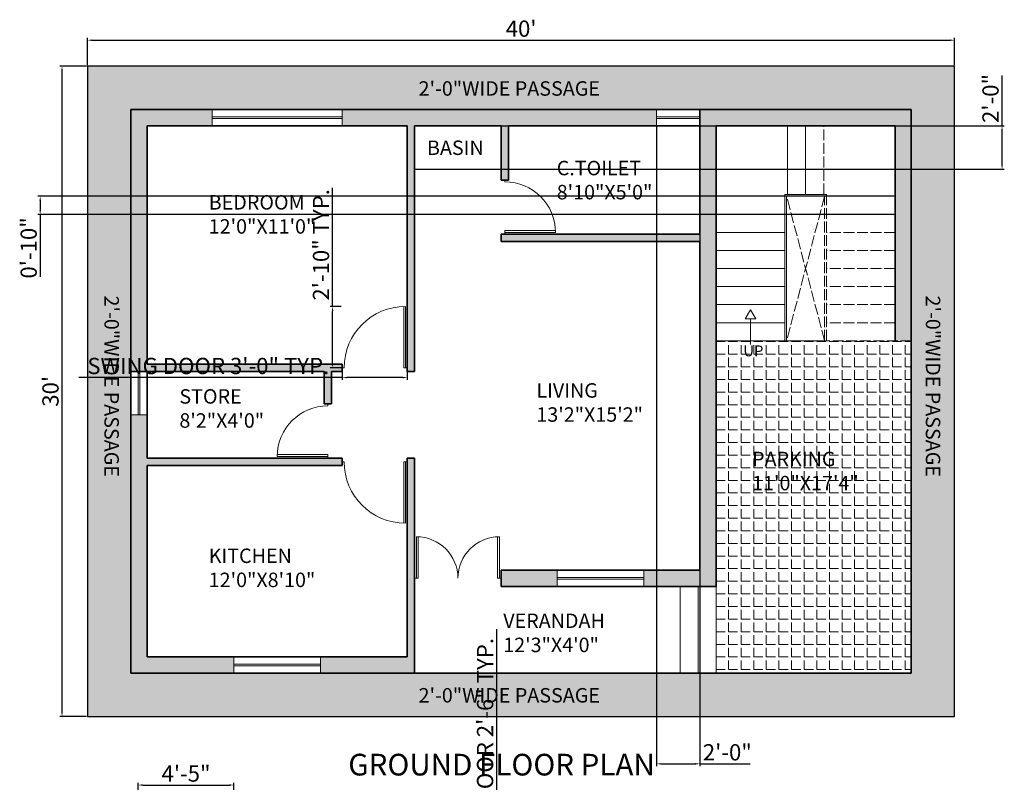
# Model space of a CAD drawing. Units: inches. Extents: x 1947 to 4744, y 610 to 1869.
# Tile 7 of 8: x 3652 to 4197, y 1446 to 1869. Entities that reach past the tile are written whole.
import ezdxf

# ---------------------------------------------------------------- set-up
doc = ezdxf.new("R2010")
doc.units = ezdxf.units.IN
doc.linetypes.add('ACAD_ISO02W100', pattern=[15, 12, -3])
for name, color, linetype, lineweight in [('A-ANNO-DIMS', 2, 'Continuous', 18), ('A-ANNO-SYMB', 2, 'Continuous', 18), ('A-ANNO-TEXT', 7, 'Continuous', 18), ('A-ANNO-TITL', 7, 'Continuous', 35), ('A-AREA-IDEN', 7, 'Continuous', 18), ('A-DOOR', 3, 'Continuous', 18), ('A-FLOR-FIXT', 9, 'Continuous', 18), ('A-FLOR-STRS', 7, 'Continuous', 18), ('A-FLOR-STRS-OVHD', 7, 'ACAD_ISO02W100', 13), ('A-GLAZ', 4, 'Continuous', 18), ('A-WALL', 7, 'Continuous', 35), ('C-PROP', 8, 'Continuous', 25)]:
    doc.layers.add(name, color=color, linetype=linetype, lineweight=lineweight)
doc.layers.add('A-FLOR-PATT', color=251, linetype='Continuous', lineweight=13, true_color=0x636466)
doc.layers.add('A-WALL-PATT', color=18, linetype='Continuous', lineweight=13, true_color=0x000000)
doc.styles.get("Standard").update_dxf_attribs({"font": 'arial.ttf'})
doc.dimstyles.new('ISO-25', dxfattribs={"dimtxt": 9, "dimasz": 2.5, "dimexe": 1.25, "dimexo": 0.625, "dimtad": 1, "dimdec": 1, "dimlunit": 3, "dimtxsty": 'Standard', "dimcen": 2.5, "dimadec": 0, "dimazin": 0, "dimtfac": 1, "dimtdec": 1, "dimtmove": 0, "dimatfit": 3, "dimfxl": 1, "dimarcsym": 0})
pattern_1 = [(0, (0, 0), (0, 6.985), [5.08, -1.905]), (90, (0, 0), (-6.985, 4e-16), [5.08, -1.905])]

# ---------------------------------------------------------------- blocks, each defined once
blk = doc.blocks.new('1')
for p, q in [((4267.36, 1627.82), (4267.36, 1650.82)), ((4268.36, 1627.82), (4268.36, 1650.82)), ((4312.36, 1627.82), (4312.36, 1650.82)), ((4313.36, 1627.82), (4313.36, 1650.82)), ((4266.36, 1627.82), (4268.36, 1627.82)), ((4314.36, 1627.82), (4312.36, 1627.82))]:
    blk.add_line(p, q)
at = {"ltscale": 0.5}
for centre, start, end in [((4267.36, 1627.82), 0, 90), ((4313.36, 1627.82), 90, 180)]:
    blk.add_arc(centre, 23, start, end, dxfattribs=at)
blk = doc.blocks.new('2')
for p, q in [((4319.45, 1679.18), (4319.45, 1713.18)), ((4320.45, 1679.18), (4320.45, 1713.18)), ((4318.45, 1679.18), (4320.45, 1679.18)), ((4353.45, 1679.18), (4354.45, 1679.18))]:
    blk.add_line(p, q)
at = {"ltscale": 0.5}
blk.add_arc((4319.45, 1679.18), 34, 0, 90, dxfattribs=at)
blk = doc.blocks.new('4')
for p, q in [((3808.6, 1693.11), (3808.6, 1721.11)), ((3809.6, 1693.11), (3809.6, 1721.11)), ((3807.6, 1693.11), (3809.6, 1693.11)), ((3836.6, 1693.11), (3837.6, 1693.11))]:
    blk.add_line(p, q)
at = {"ltscale": 0.5}
blk.add_arc((3808.6, 1693.11), 28, 0, 90, dxfattribs=at)
blk = doc.blocks.new('*D5')
at = {"layer": 'A-ANNO-DIMS', "color": 0, "lineweight": -2, "transparency": 16777216}
for p, q in [((3688.91, 1842.83), (3674.11, 1842.83)), ((3675.36, 1485.33), (3675.36, 1840.33)), ((3688.91, 1482.83), (3674.11, 1482.83))]:
    blk.add_line(p, q, dxfattribs=at)
at = {"layer": 'A-ANNO-DIMS', "color": 0, "transparency": 16777216}
for points in [[(3674.94, 1840.33), (3675.78, 1840.33), (3675.36, 1842.83)], [(3674.94, 1485.33), (3675.78, 1485.33), (3675.36, 1482.83)]]:
    blk.add_solid(points, dxfattribs=at)
at = {"layer": 'Defpoints', "color": 0, "transparency": 16777216}
for p in [(3675.36, 1842.83), (3689.53, 1842.83), (3689.53, 1482.83)]:
    blk.add_point(p, dxfattribs=at)
at = {"layer": 'A-ANNO-DIMS', "color": 0, "transparency": 16777216, "insert": (3670.14, 1662.83), "char_height": 9, "attachment_point": 5, "rotation": 90}
blk.add_mtext("30'", dxfattribs=at)
blk = doc.blocks.new('*D6')
at = {"layer": 'A-ANNO-DIMS', "color": 0, "lineweight": -2, "transparency": 16777216}
for p, q in [((3689.53, 1843.45), (3689.53, 1858.52)), ((3692.03, 1857.27), (4167.03, 1857.27)), ((4169.53, 1843.45), (4169.53, 1858.52))]:
    blk.add_line(p, q, dxfattribs=at)
at = {"layer": 'A-ANNO-DIMS', "color": 0, "transparency": 16777216}
for points in [[(3692.03, 1857.68), (3692.03, 1856.85), (3689.53, 1857.27)], [(4167.03, 1857.68), (4167.03, 1856.85), (4169.53, 1857.27)]]:
    blk.add_solid(points, dxfattribs=at)
at = {"layer": 'Defpoints', "color": 0, "transparency": 16777216}
for p in [(4169.53, 1857.27), (3689.53, 1842.83), (4169.53, 1842.83)]:
    blk.add_point(p, dxfattribs=at)
at = {"layer": 'A-ANNO-DIMS', "color": 0, "transparency": 16777216, "insert": (3929.53, 1862.49), "char_height": 9, "attachment_point": 5}
blk.add_mtext("40'", dxfattribs=at)
blk = doc.blocks.new('STAIR-DIRECTION')
blk.add_line((2.91, 14.18), (2.91, 0))
blk.add_lwpolyline([(2.91, 19.23), (0, 14.18), (5.83, 14.18)], close=True)
blk = doc.blocks.new('*D80')
at = {"layer": 'A-ANNO-DIMS', "color": 0, "lineweight": -2, "transparency": 16777216}
for p, q in [((3830.53, 1675.2), (3830.53, 1669.18)), ((3866.53, 1675.2), (3866.53, 1669.18)), ((3830.53, 1670.43), (3684.65, 1670.43)), ((3864.03, 1670.43), (3833.03, 1670.43))]:
    blk.add_line(p, q, dxfattribs=at)
at = {"layer": 'A-ANNO-DIMS', "color": 0, "transparency": 16777216}
for points in [[(3833.03, 1670.84), (3833.03, 1670.01), (3830.53, 1670.43)], [(3864.03, 1670.84), (3864.03, 1670.01), (3866.53, 1670.43)]]:
    blk.add_solid(points, dxfattribs=at)
at = {"layer": 'Defpoints', "color": 0, "transparency": 16777216}
for p in [(3830.53, 1675.83), (3866.53, 1675.83), (3830.53, 1670.43)]:
    blk.add_point(p, dxfattribs=at)
at = {"layer": 'A-ANNO-DIMS', "color": 0, "transparency": 16777216, "insert": (3756.34, 1675.71), "char_height": 9, "attachment_point": 5}
blk.add_mtext('SWING DOOR 3\'-0" TYP.', dxfattribs=at)
blk = doc.blocks.new('*D81')
at = {"layer": 'A-ANNO-DIMS', "color": 0, "lineweight": -2, "transparency": 16777216}
for p, q in [((3825.13, 1709.83), (3825.13, 1775.58)), ((3829.91, 1709.83), (3823.88, 1709.83)), ((3825.13, 1678.33), (3825.13, 1707.33)), ((3829.91, 1675.83), (3823.88, 1675.83))]:
    blk.add_line(p, q, dxfattribs=at)
at = {"layer": 'A-ANNO-DIMS', "color": 0, "transparency": 16777216}
for points in [[(3824.71, 1707.33), (3825.55, 1707.33), (3825.13, 1709.83)], [(3824.71, 1678.33), (3825.55, 1678.33), (3825.13, 1675.83)]]:
    blk.add_solid(points, dxfattribs=at)
at = {"layer": 'Defpoints', "color": 0, "transparency": 16777216}
for p in [(3825.13, 1709.83), (3830.53, 1709.83), (3830.53, 1675.83)]:
    blk.add_point(p, dxfattribs=at)
at = {"layer": 'A-ANNO-DIMS', "color": 0, "transparency": 16777216, "insert": (3819.91, 1743.96), "char_height": 9, "attachment_point": 5, "rotation": 90}
blk.add_mtext('2\'-10" TYP.', dxfattribs=at)
blk = doc.blocks.new('*D82')
at = {"layer": 'A-ANNO-DIMS', "color": 0, "lineweight": -2, "transparency": 16777216}
for p, q in [((3916.03, 1381.79), (3916.03, 1531.18)), ((3919.91, 1381.79), (3914.78, 1381.79)), ((3916.03, 1354.29), (3916.03, 1379.29)), ((3919.91, 1351.79), (3914.78, 1351.79))]:
    blk.add_line(p, q, dxfattribs=at)
at = {"layer": 'A-ANNO-DIMS', "color": 0, "transparency": 16777216}
for points in [[(3915.61, 1379.29), (3916.45, 1379.29), (3916.03, 1381.79)], [(3915.61, 1354.29), (3916.45, 1354.29), (3916.03, 1351.79)]]:
    blk.add_solid(points, dxfattribs=at)
at = {"layer": 'Defpoints', "color": 0, "transparency": 16777216}
for p in [(3916.03, 1381.79), (3920.53, 1381.79), (3920.53, 1351.79)]:
    blk.add_point(p, dxfattribs=at)
at = {"layer": 'A-ANNO-DIMS', "color": 0, "transparency": 16777216, "insert": (3910.75, 1457.73), "char_height": 9, "attachment_point": 5, "rotation": 90}
blk.add_mtext('SINGLE DOOR 2\'-6" TYP.', dxfattribs=at)
blk = doc.blocks.new('*D98')
at = {"layer": 'A-ANNO-DIMS', "color": 0, "lineweight": -2, "transparency": 16777216}
for p, q in [((4135.91, 1770.83), (3662.03, 1770.83)), ((3663.28, 1768.33), (3663.28, 1763.33)), ((4135.91, 1760.83), (3662.03, 1760.83)), ((3663.28, 1760.83), (3663.28, 1726.16))]:
    blk.add_line(p, q, dxfattribs=at)
at = {"layer": 'A-ANNO-DIMS', "color": 0, "transparency": 16777216}
for points in [[(3662.86, 1768.33), (3663.7, 1768.33), (3663.28, 1770.83)], [(3662.86, 1763.33), (3663.7, 1763.33), (3663.28, 1760.83)]]:
    blk.add_solid(points, dxfattribs=at)
at = {"layer": 'Defpoints', "color": 0, "transparency": 16777216}
for p in [(4136.53, 1770.83), (3663.28, 1760.83), (4136.53, 1760.83)]:
    blk.add_point(p, dxfattribs=at)
at = {"layer": 'A-ANNO-DIMS', "color": 0, "transparency": 16777216, "insert": (3658.06, 1742.24), "char_height": 9, "attachment_point": 5, "rotation": 90}
blk.add_mtext('0\'-10"', dxfattribs=at)
blk = doc.blocks.new('*D100')
at = {"layer": 'A-ANNO-DIMS', "color": 0, "lineweight": -2, "transparency": 16777216}
for p, q in [((4195.78, 1809.83), (4195.78, 1837.66)), ((3871.16, 1809.83), (4197.03, 1809.83)), ((4195.78, 1788.33), (4195.78, 1807.33)), ((3871.16, 1785.83), (4197.03, 1785.83))]:
    blk.add_line(p, q, dxfattribs=at)
at = {"layer": 'A-ANNO-DIMS', "color": 0, "transparency": 16777216}
for points in [[(4195.36, 1807.33), (4196.2, 1807.33), (4195.78, 1809.83)], [(4195.36, 1788.33), (4196.2, 1788.33), (4195.78, 1785.83)]]:
    blk.add_solid(points, dxfattribs=at)
at = {"layer": 'Defpoints', "color": 0, "transparency": 16777216}
for p in [(3870.53, 1809.83), (4195.78, 1809.83), (3870.53, 1785.83)]:
    blk.add_point(p, dxfattribs=at)
at = {"layer": 'A-ANNO-DIMS', "color": 0, "transparency": 16777216, "insert": (4190.56, 1824.99), "char_height": 9, "attachment_point": 5, "rotation": 90}
blk.add_mtext('2\'-0"', dxfattribs=at)
blk = doc.blocks.new('*D108')
at = {"layer": 'A-ANNO-DIMS', "color": 0, "lineweight": -2, "transparency": 16777216}
for p, q in [((3717.53, 1113.41), (3717.53, 1446.09)), ((3720.03, 1444.84), (3768.03, 1444.84)), ((3770.53, 1113.41), (3770.53, 1446.09))]:
    blk.add_line(p, q, dxfattribs=at)
at = {"layer": 'A-ANNO-DIMS', "color": 0, "transparency": 16777216}
for points in [[(3720.03, 1445.26), (3720.03, 1444.42), (3717.53, 1444.84)], [(3768.03, 1445.26), (3768.03, 1444.42), (3770.53, 1444.84)]]:
    blk.add_solid(points, dxfattribs=at)
at = {"layer": 'Defpoints', "color": 0, "transparency": 16777216}
for p in [(3770.53, 1444.84), (3717.53, 1112.79), (3770.53, 1112.79)]:
    blk.add_point(p, dxfattribs=at)
at = {"layer": 'A-ANNO-DIMS', "color": 0, "transparency": 16777216, "insert": (3744.03, 1450.04), "char_height": 9, "attachment_point": 5}
blk.add_mtext('4\'-5"', dxfattribs=at)
blk = doc.blocks.new('*D112')
at = {"layer": 'A-ANNO-DIMS', "color": 0, "lineweight": -2, "transparency": 16777216}
for p, q in [((4004.53, 1809.2), (4004.53, 1455.33)), ((4028.53, 1809.2), (4028.53, 1455.33)), ((4007.03, 1456.58), (4026.03, 1456.58)), ((4028.53, 1456.58), (4056.36, 1456.58))]:
    blk.add_line(p, q, dxfattribs=at)
at = {"layer": 'A-ANNO-DIMS', "color": 0, "transparency": 16777216}
for points in [[(4007.03, 1456.99), (4007.03, 1456.16), (4004.53, 1456.58)], [(4026.03, 1456.99), (4026.03, 1456.16), (4028.53, 1456.58)]]:
    blk.add_solid(points, dxfattribs=at)
at = {"layer": 'Defpoints', "color": 0, "transparency": 16777216}
for p in [(4004.53, 1809.83), (4028.53, 1809.83), (4028.53, 1456.58)]:
    blk.add_point(p, dxfattribs=at)
at = {"layer": 'A-ANNO-DIMS', "color": 0, "transparency": 16777216, "insert": (4043.69, 1461.8), "char_height": 9, "attachment_point": 5}
blk.add_mtext('2\'-0"', dxfattribs=at)

msp = doc.modelspace()

# ---------------------------------------------------------------- hatches: boundary and pattern name
at = {"layer": 'A-FLOR-PATT'}
h = msp.add_hatch(dxfattribs=at)
h.set_pattern_fill('ANGLE', color=256)
h.set_pattern_definition(pattern_1)
h.paths.add_polyline_path([(3689.53, 1842.83), (3689.53, 1482.83), (4169.53, 1482.83), (4169.53, 1842.83)])
h.paths.add_polyline_path([(4145.53, 1818.83), (4145.53, 1506.83), (3713.53, 1506.83), (3713.53, 1818.83)], flags=16)
h.paths.add_polyline_path([(4136.53, 1809.83), (4136.53, 1690.83), (4097.53, 1690.83), (4037.53, 1690.83), (4037.53, 1554.83), (3918.53, 1554.83), (3918.53, 1563.83), (4028.53, 1563.83), (4028.53, 1745.83), (3918.53, 1745.83), (3918.53, 1749.83), (4028.53, 1749.83), (4028.53, 1809.83), (3922.53, 1809.83), (3922.53, 1779.83), (3918.53, 1779.83), (3918.53, 1785.83), (3870.53, 1785.83), (3870.53, 1673.83), (3866.53, 1673.83), (3866.53, 1809.83), (3722.53, 1809.83), (3722.53, 1677.83), (3830.53, 1677.83), (3830.53, 1673.83), (3824.53, 1673.83), (3824.53, 1655.83), (3820.53, 1655.83), (3820.53, 1673.83), (3722.53, 1673.83), (3722.53, 1625.83), (3830.53, 1625.83), (3830.53, 1621.83), (3722.53, 1621.83), (3722.53, 1515.83), (3818.53, 1515.83), (3818.53, 1510.83), (3770.53, 1510.83), (3770.53, 1515.83), (3722.53, 1515.83), (3722.53, 1621.83), (3830.53, 1621.83), (3830.53, 1625.83), (3722.53, 1625.83), (3722.53, 1649.83), (3717.53, 1649.83), (3717.53, 1673.83), (3820.53, 1673.83), (3820.53, 1655.83), (3824.53, 1655.83), (3824.53, 1673.83), (3830.53, 1673.83), (3830.53, 1677.83), (3722.53, 1677.83), (3722.53, 1809.83), (3758.53, 1809.83), (3758.53, 1814.83), (3830.53, 1814.83), (3830.53, 1809.83), (3866.53, 1809.83), (3866.53, 1673.83), (3870.53, 1673.83), (3870.53, 1809.83), (3918.53, 1809.83), (3918.53, 1779.83), (3922.53, 1779.83), (3922.53, 1809.83), (4004.53, 1809.83), (4004.53, 1814.83), (4028.53, 1814.83), (4028.53, 1749.83), (3918.53, 1749.83), (3918.53, 1745.83), (4028.53, 1745.83), (4028.53, 1563.83), (3997.53, 1563.83), (3997.53, 1554.83), (4037.53, 1554.83), (4037.53, 1809.83)], flags=0)
h.paths.add_polyline_path([(4076.53, 1770.83), (4097.53, 1770.83), (4097.53, 1690.83), (4087.03, 1730.83), (4076.53, 1690.83)], flags=0)
h.paths.add_polyline_path([(3875.22, 1789.16), (3914.67, 1789.16), (3914.67, 1806.24), (3875.22, 1806.24)], flags=8)
h.paths.add_polyline_path([(3870.52, 1485.98), (3983.52, 1485.98), (3983.52, 1503.06), (3870.52, 1503.06)], flags=24)
h.paths.add_polyline_path([(3694.29, 1718.11), (3694.29, 1605.12), (3711.37, 1605.12), (3711.37, 1718.11)], flags=24)
h.paths.add_polyline_path([(4149.02, 1718.11), (4149.02, 1605.12), (4166.11, 1605.12), (4166.11, 1718.11)], flags=24)
h.paths.add_polyline_path([(3870.52, 1821.98), (3983.52, 1821.98), (3983.52, 1839.06), (3870.52, 1839.06)], flags=24)
h.paths.add_polyline_path([(3916.25, 1513.88), (3987.81, 1513.88), (3987.81, 1544.29), (3916.25, 1544.29)], flags=8)
h.paths.add_polyline_path([(4054.04, 1603.48), (4115.91, 1603.48), (4115.91, 1633.9), (4054.04, 1633.9)], flags=8)
h.paths.add_polyline_path([(3737.61, 1638.13), (3787.69, 1638.13), (3787.69, 1668.55), (3737.61, 1668.55)], flags=8)
h.paths.add_polyline_path([(3946.51, 1764.58), (4002.96, 1764.58), (4002.96, 1795), (3946.51, 1795)], flags=8)
h.paths.add_polyline_path([(3934.6, 1641.45), (3996.46, 1641.45), (3996.46, 1671.86), (3934.6, 1671.86)], flags=8)
h.paths.add_polyline_path([(3753.2, 1549.89), (3815.06, 1549.89), (3815.06, 1580.3), (3753.2, 1580.3)], flags=8)
h.paths.add_polyline_path([(3753.2, 1745.59), (3817.45, 1745.59), (3817.45, 1776), (3753.2, 1776)], flags=8)
h = msp.add_hatch(dxfattribs=at)
h.set_pattern_fill('ANGLE', color=256)
h.set_pattern_definition(pattern_1)
h.paths.add_polyline_path([(4145.53, 1690.83), (4097.53, 1690.83), (4037.53, 1690.83), (4037.53, 1554.83), (4037.53, 1506.83), (4145.53, 1506.83)])
h.paths.add_polyline_path([(4051, 1678.84), (4065.33, 1678.84), (4065.33, 1691.65), (4051, 1691.65)], flags=9)
h.paths.add_polyline_path([(4054.04, 1603.48), (4115.91, 1603.48), (4115.91, 1633.9), (4054.04, 1633.9)], flags=24)
at = {"layer": 'A-WALL-PATT'}
h = msp.add_hatch(color=256, dxfattribs=at)
h.dxf.hatch_style = 1
h.paths.add_polyline_path([(3758.53, 1818.83), (3713.53, 1818.83), (3713.53, 1673.83), (3820.53, 1673.83), (3820.53, 1655.83), (3824.53, 1655.83), (3824.53, 1673.83), (3830.53, 1673.83), (3830.53, 1677.83), (3722.53, 1677.83), (3722.53, 1809.83), (3758.53, 1809.83)])
h.paths.add_polyline_path([(4004.53, 1818.83), (3830.53, 1818.83), (3830.53, 1809.83), (3866.53, 1809.83), (3866.53, 1673.83), (3870.53, 1673.83), (3870.53, 1809.83), (3918.53, 1809.83), (3918.53, 1779.83), (3922.53, 1779.83), (3922.53, 1809.83), (4004.53, 1809.83)])
h.paths.add_polyline_path([(4037.53, 1809.83), (4136.53, 1809.83), (4136.53, 1690.83), (4145.53, 1690.83), (4145.53, 1818.83), (4028.53, 1818.83), (4028.53, 1749.83), (3918.53, 1749.83), (3918.53, 1745.83), (4028.53, 1745.83), (4028.53, 1563.83), (3997.53, 1563.83), (3997.53, 1554.83), (4037.53, 1554.83)])
h.paths.add_polyline_path([(3870.53, 1625.83), (3866.53, 1625.83), (3866.53, 1515.83), (3818.53, 1515.83), (3818.53, 1506.83), (3870.53, 1506.83)])
h.paths.add_polyline_path([(3770.53, 1515.83), (3722.53, 1515.83), (3722.53, 1621.83), (3830.53, 1621.83), (3830.53, 1625.83), (3722.53, 1625.83), (3722.53, 1649.83), (3713.53, 1649.83), (3713.53, 1506.83), (3770.53, 1506.83)])
h.paths.add_polyline_path([(3949.53, 1563.83), (3918.53, 1563.83), (3918.53, 1554.83), (3949.53, 1554.83)])

# ---------------------------------------------------------------- linework, layer by layer
at = {"layer": 'A-FLOR-FIXT'}
msp.add_line((3918.53, 1785.83), (3870.53, 1785.83), dxfattribs=at)
at = {"layer": 'A-FLOR-STRS'}
for p, q in [((4077.03, 1771.83), (4077.03, 1809.83)), ((4087.03, 1771.83), (4087.03, 1809.83)), ((4098.53, 1771.83), (4075.53, 1771.83)), ((4075.53, 1690.83), (4075.53, 1771.83)), ((4075.53, 1770.83), (4037.53, 1770.83)), ((4097.53, 1770.83), (4076.53, 1770.83)), ((4076.53, 1690.83), (4076.53, 1770.83)), ((4075.53, 1760.83), (4037.53, 1760.83)), ((4075.53, 1750.83), (4037.53, 1750.83)), ((4075.53, 1740.83), (4037.53, 1740.83)), ((4075.53, 1730.83), (4037.53, 1730.83)), ((4075.53, 1720.83), (4037.53, 1720.83)), ((4075.53, 1710.83), (4037.53, 1710.83)), ((4075.53, 1700.83), (4037.53, 1700.83)), ((4097.53, 1690.83), (4037.53, 1690.83)), ((4017.53, 1554.83), (4017.53, 1506.83)), ((4027.53, 1554.83), (4027.53, 1506.83)), ((4037.53, 1554.83), (4037.53, 1506.83))]:
    msp.add_line(p, q, dxfattribs=at)
at = {"layer": 'A-FLOR-STRS-OVHD', "ltscale": 0.5}
for p, q in [((4097.03, 1771.83), (4097.03, 1809.83)), ((4098.53, 1690.83), (4098.53, 1771.83)), ((4097.53, 1770.83), (4076.53, 1690.83)), ((4097.53, 1690.83), (4076.53, 1770.83)), ((4097.53, 1690.83), (4097.53, 1770.83)), ((4136.53, 1770.83), (4098.53, 1770.83)), ((4136.53, 1760.83), (4098.53, 1760.83)), ((4136.53, 1750.83), (4098.53, 1750.83)), ((4136.53, 1740.83), (4098.53, 1740.83)), ((4136.53, 1730.83), (4098.53, 1730.83)), ((4136.53, 1720.83), (4098.53, 1720.83)), ((4136.53, 1710.83), (4098.53, 1710.83)), ((4136.53, 1700.83), (4098.53, 1700.83)), ((4145.53, 1690.83), (4097.53, 1690.83))]:
    msp.add_line(p, q, dxfattribs=at)
at = {"layer": 'A-GLAZ'}
for p, q in [((3758.53, 1809.83), (3758.53, 1818.83)), ((3830.53, 1809.83), (3830.53, 1818.83)), ((4004.53, 1809.83), (4004.53, 1818.83)), ((3830.53, 1814.83), (3758.53, 1814.83)), ((3830.53, 1813.83), (3758.53, 1813.83)), ((4028.53, 1814.83), (4004.53, 1814.83)), ((4028.53, 1813.83), (4004.53, 1813.83)), ((3717.53, 1673.83), (3717.53, 1649.83)), ((3718.53, 1673.83), (3718.53, 1649.83)), ((3722.53, 1649.83), (3713.53, 1649.83)), ((3949.53, 1554.83), (3949.53, 1563.83)), ((3997.53, 1559.83), (3949.53, 1559.83)), ((3997.53, 1554.83), (3997.53, 1563.83)), ((3997.53, 1558.83), (3949.53, 1558.83)), ((3770.53, 1506.83), (3770.53, 1515.83)), ((3818.53, 1506.83), (3818.53, 1515.83)), ((3818.53, 1511.83), (3770.53, 1511.83)), ((3818.53, 1510.83), (3770.53, 1510.83))]:
    msp.add_line(p, q, dxfattribs=at)
at = {"layer": 'A-WALL'}
for p, q in [((4145.53, 1818.83), (3713.53, 1818.83)), ((3713.53, 1818.83), (3713.53, 1506.83)), ((4028.53, 1749.83), (4028.53, 1818.83)), ((4145.53, 1506.83), (4145.53, 1818.83)), ((3722.53, 1809.83), (3722.53, 1677.83)), ((3866.53, 1809.83), (3722.53, 1809.83)), ((3866.53, 1809.83), (3866.53, 1673.83)), ((3870.53, 1809.83), (3870.53, 1673.83)), ((3918.53, 1809.83), (3870.53, 1809.83)), ((3918.53, 1779.83), (3918.53, 1809.83)), ((3922.53, 1779.83), (3922.53, 1809.83)), ((4028.53, 1809.83), (3922.53, 1809.83)), ((4136.53, 1809.83), (4037.53, 1809.83)), ((4037.53, 1554.83), (4037.53, 1809.83)), ((4136.53, 1690.83), (4136.53, 1809.83)), ((3922.53, 1779.83), (3918.53, 1779.83)), ((4028.53, 1749.83), (3918.53, 1749.83)), ((3918.53, 1745.83), (3918.53, 1749.83)), ((3918.53, 1745.83), (4028.53, 1745.83)), ((4028.53, 1563.83), (4028.53, 1745.83)), ((3820.53, 1673.83), (3713.53, 1673.83)), ((3830.53, 1677.83), (3722.53, 1677.83)), ((3722.53, 1673.83), (3722.53, 1625.83)), ((3820.53, 1673.83), (3820.53, 1655.83)), ((3824.53, 1673.83), (3824.53, 1655.83)), ((3830.53, 1673.83), (3824.53, 1673.83)), ((3830.53, 1677.83), (3830.53, 1673.83)), ((3870.53, 1673.83), (3866.53, 1673.83)), ((3824.53, 1655.83), (3820.53, 1655.83)), ((3830.53, 1625.83), (3722.53, 1625.83)), ((3830.53, 1625.83), (3830.53, 1621.83)), ((3870.53, 1625.83), (3866.53, 1625.83)), ((3866.53, 1625.83), (3866.53, 1515.83)), ((3870.53, 1625.83), (3870.53, 1506.83)), ((3830.53, 1621.83), (3722.53, 1621.83)), ((3722.53, 1621.83), (3722.53, 1515.83)), ((3918.53, 1563.83), (4028.53, 1563.83)), ((3918.53, 1563.83), (3918.53, 1554.83)), ((3918.53, 1554.83), (4037.53, 1554.83)), ((3722.53, 1515.83), (3866.53, 1515.83)), ((3713.53, 1506.83), (4145.53, 1506.83))]:
    msp.add_line(p, q, dxfattribs=at)
at = {"layer": 'C-PROP'}
msp.add_lwpolyline([(3689.53, 1482.83), (4169.53, 1482.83), (4169.53, 1842.83), (3689.53, 1842.83)], close=True, dxfattribs=at)

# ---------------------------------------------------------------- block references
at = {"layer": 'A-ANNO-SYMB'}
msp.add_blockref('STAIR-DIRECTION', (4053.62, 1688.75), dxfattribs=at)
at = {"layer": 'A-DOOR', "xscale": -1, "rotation": 270}
msp.add_blockref('4', (2227.42, -2057.77), dxfattribs=at)
at = {"layer": 'A-DOOR', "xscale": -1}
msp.add_blockref('2', (8184.98, -3.36), dxfattribs=at)
at = {"layer": 'A-DOOR'}
for name, p, rotation in [('4', (5515.64, -2181.77), 90), ('2', (8184.98, 3303.01), 180)]:
    msp.add_blockref(name, p, dxfattribs=dict(at, rotation=rotation))
msp.add_blockref('1', (-395.83, -68.5), dxfattribs=at)

# ---------------------------------------------------------------- texts
at = {"layer": 'A-ANNO-TEXT', "attachment_point": 1}
for s, insert, char_height in [('{\\fTimes New Roman|b0|i0|c0|p18;BASIN}', (3877.42, 1801.71), 8), ('{\\fTimes New Roman|b0|i0|c0|p18;UP}', (4052.55, 1688.25), 6)]:
    msp.add_mtext_dynamic_manual_height_columns(s, width=158.3328, gutter_width=12.5, heights=[0], dxfattribs=dict(at, insert=insert, char_height=char_height))
at = {"layer": 'A-ANNO-TITL', "insert": (3833.83, 1462.13), "char_height": 12, "attachment_point": 1}
msp.add_mtext_dynamic_manual_height_columns('{\\fTimes New Roman|b0|i0|c0|p18;GROUND FLOOR PLAN}', width=253.4596, gutter_width=12.5, heights=[0], dxfattribs=at)
at = {"layer": 'A-AREA-IDEN', "char_height": 8, "attachment_point": 1}
for s, width, heights, insert in [('{\\fTimes New Roman|b0|i0|c0|p18;2\'-0"WIDE PASSAGE}', 158.3328, [0], (3872.77, 1834.53)), ('{\\fTimes New Roman|b0|i0|c0|p18;C.TOILET\\P8\'10"X5\'0"}', 64.3566, [21.47], (3949.23, 1790.47)), ('{\\fTimes New Roman|b0|i0|c0|p18;BEDROOM\\P12\'0"X11\'0"}', 64.3566, [0], (3756.58, 1771.48)), ('{\\fTimes New Roman|b0|i0|c0|p18;STORE\\P8\'2"X4\'0"}', 64.3566, [21.47], (3740.35, 1664.02)), ('{\\fTimes New Roman|b0|i0|c0|p18;LIVING\\P13\'2"X15\'2"}', 64.3566, [21.47], (3937.98, 1667.33)), ('{\\fTimes New Roman|b0|i0|c0|p18;PARKING\\P11\'0"X17\'4"}', 64.3566, [0], (4057.42, 1629.37)), ('{\\fTimes New Roman|b0|i0|c0|p18;KITCHEN\\P12\'0"X8\'10"}', 64.3566, [0], (3756.58, 1575.78)), ('{\\fTimes New Roman|b0|i0|c0|p18;VERANDAH\\P12\'3"X4\'0"}', 64.3566, [0], (3919.64, 1539.77)), ('{\\fTimes New Roman|b0|i0|c0|p18;2\'-0"WIDE PASSAGE}', 158.3328, [0], (3872.77, 1498.53))]:
    msp.add_mtext_dynamic_manual_height_columns(s, width=width, gutter_width=12.5, heights=heights, dxfattribs=dict(at, insert=insert))
at = {"layer": 'A-AREA-IDEN', "char_height": 8, "attachment_point": 1, "rotation": 270}
for insert in [(3706.84, 1715.86), (4161.58, 1715.86)]:
    msp.add_mtext_dynamic_manual_height_columns('{\\fTimes New Roman|b0|i0|c0|p18;2\'-0"WIDE PASSAGE}', width=158.3328, gutter_width=12.5, heights=[0], dxfattribs=dict(at, insert=insert))

# ---------------------------------------------------------------- dimensions: what is measured, and where the dimension line sits
at = {"layer": 'A-ANNO-DIMS'}
for base, p1, p2, override, picture, middle in [((4169.53, 1857.27), (3689.53, 1842.83), (4169.53, 1842.83), {"dimclrd": 0, "dimclre": 0, "dimclrt": 0}, '*D6', (3929.53, 1862.49)), ((4028.53, 1456.58), (4004.53, 1809.83), (4028.53, 1809.83), {"dimdec": 1, "dimlfac": 1, "dimrnd": 0, "dimzin": 1, "dimdsep": 46, "dimlunit": 4, "dimfrac": 2}, '*D112', (4043.69, 1461.8)), ((3770.53, 1444.84), (3717.53, 1112.79), (3770.53, 1112.79), {"dimdec": 1, "dimlfac": 1, "dimrnd": 0, "dimzin": 1, "dimdsep": 46, "dimlunit": 4, "dimfrac": 2}, '*D108', (3744.03, 1450.04))]:
    dim = msp.add_linear_dim(base=base, p1=p1, p2=p2, dimstyle='ISO-25', override=override, dxfattribs=at)
    dim.commit()
    dim.dimension.update_dxf_attribs({"geometry": picture, "text_midpoint": middle})
for base, p1, p2, override, picture, middle in [((3675.36, 1842.83), (3689.53, 1482.83), (3689.53, 1842.83), {"dimclrd": 0, "dimclre": 0, "dimclrt": 0}, '*D5', (3670.14, 1662.83)), ((4195.78, 1809.83), (3870.53, 1785.83), (3870.53, 1809.83), {"dimdec": 1, "dimlfac": 1, "dimrnd": 0, "dimzin": 1, "dimdsep": 46, "dimlunit": 4, "dimfrac": 2}, '*D100', (4190.56, 1824.99)), ((3663.28, 1760.83), (4136.53, 1770.83), (4136.53, 1760.83), {"dimdec": 1, "dimlfac": 1, "dimrnd": 0, "dimzin": 1, "dimdsep": 46, "dimlunit": 4, "dimfrac": 2}, '*D98', (3658.06, 1742.24))]:
    dim = msp.add_linear_dim(base=base, p1=p1, p2=p2, angle=90, dimstyle='ISO-25', override=override, dxfattribs=at)
    dim.commit()
    dim.dimension.update_dxf_attribs({"geometry": picture, "text_midpoint": middle})
for base, p1, p2, angle, text, picture, middle in [((3825.13, 1709.83), (3830.53, 1675.83), (3830.53, 1709.83), 90, '<> TYP.', '*D81', (3819.91, 1743.96)), ((3830.53, 1670.43), (3866.53, 1675.83), (3830.53, 1675.83), 180, 'SWING DOOR <> TYP.', '*D80', (3756.34, 1675.71)), ((3916.03, 1381.79), (3920.53, 1351.79), (3920.53, 1381.79), 90, 'SINGLE DOOR <> TYP.', '*D82', (3910.75, 1457.73))]:
    dim = msp.add_linear_dim(base=base, p1=p1, p2=p2, angle=angle, text=text, dimstyle='ISO-25', override={"dimdec": 1, "dimlfac": 1, "dimrnd": 0, "dimzin": 1, "dimdsep": 46, "dimlunit": 4, "dimfrac": 2}, dxfattribs=at)
    dim.commit()
    dim.dimension.update_dxf_attribs({"geometry": picture, "text_midpoint": middle})

doc.saveas('drawing.dxf')
